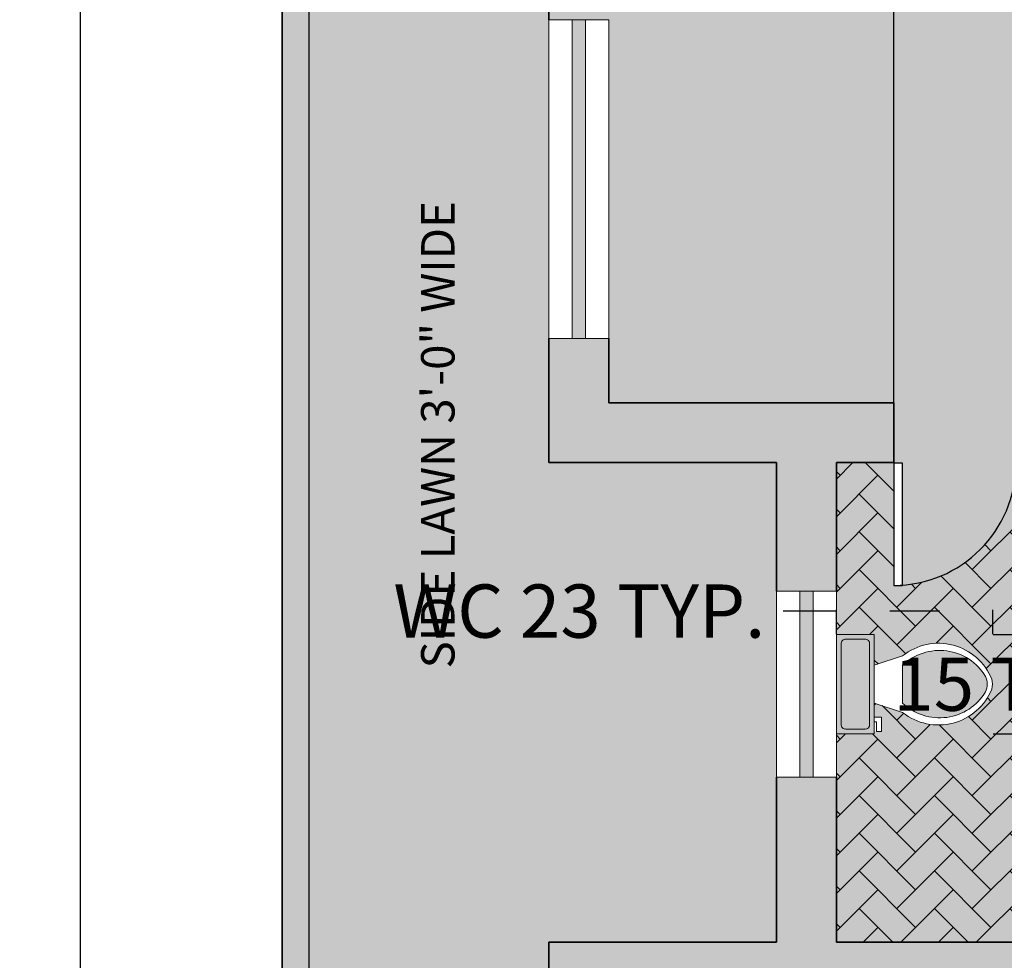
# Model space of a CAD drawing. Units: inches. Extents: x 389 to 971, y 148 to 870.
# Tile 8 of 14: x 389 to 537, y 558 to 699. Entities that reach past the tile are written whole.
import ezdxf

# ---------------------------------------------------------------- set-up
doc = ezdxf.new("R2010")
doc.units = ezdxf.units.IN
doc.header["$MEASUREMENT"] = 0
for name, color, linetype, lineweight in [('A-ANNO-DIMS', 2, 'Continuous', 18), ('A-ANNO-TEXT', 7, 'Continuous', 18), ('A-DOOR', 4, 'Continuous', 25), ('A-FLOR-BASE-PATT', 8, 'Continuous', 13), ('A-FLOR-FIXT', 8, 'Continuous', 18), ('A-FLOR-FIXT-PATT', 9, 'Continuous', 13), ('A-FLOR-PATT', 9, 'Continuous', 13), ('A-GLAZ', 4, 'Continuous', 18), ('A-WALL', 7, 'Continuous', 35), ('C-PROP', 7, 'Continuous', 35), ('L-GRND-BASE-PATT', 8, 'Continuous', 13), ('L-WALL', 7, 'Continuous', 30)]:
    doc.layers.add(name, color=color, linetype=linetype, lineweight=lineweight)
for name, color, linetype, lineweight, true_color in [('A-GLAZ-PATT', 251, 'Continuous', 13, 0x6d5f6c), ('A-WALL-PATT', 18, 'Continuous', 13, 0x000000), ('L-GRND-PATT', 39, 'Continuous', 13, 0x603913)]:
    doc.layers.add(name, color=color, linetype=linetype, lineweight=lineweight, true_color=true_color)
doc.styles.get("Standard").update_dxf_attribs({"font": 'arial.ttf'})
doc.dimstyles.get("Standard").update_dxf_attribs({"dimtxt": 8, "dimasz": 8, "dimexe": 0.18, "dimexo": 0.0625, "dimgap": 0.09, "dimtad": 0, "dimtih": 1, "dimtoh": 1, "dimdec": 0, "dimzin": 0, "dimdsep": 46, "dimlunit": 3, "dimtxsty": 'Standard', "dimcen": 0.09, "dimadec": 0, "dimazin": 0, "dimtfac": 1, "dimtdec": 0, "dimtofl": 0, "dimtmove": 0, "dimatfit": 3, "dimfxl": 1, "dimtolj": 1, "dimtzin": 0, "dimarcsym": 0})

# ---------------------------------------------------------------- blocks, each defined once
blk = doc.blocks.new('*U4')
for p, q in [((0, 0), (0, 6)), ((24, 0), (24, 6))]:
    blk.add_line(p, q)
blk.add_lwpolyline([(0, 0), (0, -24), (1.75, -24), (1.75, 0)], close=True)
blk.add_arc((0, 0), 24, 270, 0)
blk = doc.blocks.new('Toilet - top')
for p, q in [((9.5, -6), (9.5, -2)), ((-8, -8.5), (-8, -8)), ((-7, -8), (-7, -9.5)), ((-4, -8), (-6, -14)), ((4, -8), (6, -14)), ((-10, -8.5), (-8, -8.5)), ((-10, -9.5), (-10, -8.5)), ((-7, -9.5), (-10, -9.5)), ((4, -14), (-4, -14))]:
    blk.add_line(p, q)
blk.add_lwpolyline([(10.5, -8), (10.5, 0), (-10.5, 0), (-10.5, -8)], close=True)
for points in [[(-9.5, -2), (-9.5, -6)], [(8.5, -1), (-8.5, -1)], [(-8.5, -7), (8.5, -7)]]:
    blk.add_lwpolyline(points)
for centre, radius, start, end in [((-8.62, -1.88), 0.884, 81.8699, 188.1301), ((8.62, -1.88), 0.884, 351.8699, 98.1301), ((-8.62, -6.12), 0.884, 171.8699, 278.1301), ((8.62, -6.12), 0.884, 261.8699, 8.1301), ((3.52, -21.58), 12.17, 141.4691, 247.9714), ((4.2, -21.82), 11.33, 136.3677, 238.9468), ((-3.52, -21.58), 12.17, 292.0284, 38.5307), ((-4.2, -21.82), 11.33, 301.053, 43.6321), ((0, -27.88), 4, 245.7318, 294.2682), ((0, -29), 4, 254.8605, 285.1395)]:
    blk.add_arc(centre, radius, start, end)
blk = doc.blocks.new('*D26')
at = {"layer": 'A-ANNO-DIMS', "color": 0, "lineweight": -2, "transparency": 16777216}
for p, q in [((511.39, 610.36), (503.39, 610.36)), ((511.39, 606.91), (511.39, 610.54)), ((526.83, 610.36), (519.39, 610.36)), ((534.83, 606.91), (534.83, 610.54))]:
    blk.add_line(p, q, dxfattribs=at)
at = {"layer": 'A-ANNO-DIMS', "color": 0, "transparency": 16777216}
for points in [[(519.39, 611.69), (519.39, 609.03), (511.39, 610.36)], [(526.83, 611.69), (526.83, 609.03), (534.83, 610.36)]]:
    blk.add_solid(points, dxfattribs=at)
at = {"layer": 'Defpoints', "color": 0, "transparency": 16777216}
for p in [(511.39, 610.36), (511.39, 606.84), (534.83, 606.84)]:
    blk.add_point(p, dxfattribs=at)
at = {"layer": 'A-ANNO-DIMS', "color": 0, "transparency": 16777216, "insert": (472.8, 610.36), "char_height": 8, "attachment_point": 5}
blk.add_mtext('\\A1;WC 23 TYP.', dxfattribs=at)
blk = doc.blocks.new('*D27')
at = {"layer": 'A-ANNO-DIMS', "color": 0, "lineweight": -2, "transparency": 16777216}
for p, q in [((538.35, 614.84), (538.35, 622.84)), ((534.89, 606.84), (538.53, 606.84)), ((534.89, 591.95), (538.53, 591.95)), ((538.35, 583.95), (538.35, 575.95))]:
    blk.add_line(p, q, dxfattribs=at)
at = {"layer": 'A-ANNO-DIMS', "color": 0, "transparency": 16777216}
for points in [[(537.01, 614.84), (539.68, 614.84), (538.35, 606.84)], [(537.01, 583.95), (539.68, 583.95), (538.35, 591.95)]]:
    blk.add_solid(points, dxfattribs=at)
at = {"layer": 'Defpoints', "color": 0, "transparency": 16777216}
for p in [(534.83, 606.84), (538.35, 606.84), (534.83, 591.95)]:
    blk.add_point(p, dxfattribs=at)
at = {"layer": 'A-ANNO-DIMS', "color": 0, "transparency": 16777216, "insert": (538.35, 599.39), "char_height": 8, "attachment_point": 5}
blk.add_mtext('\\A1;15 TYP.', dxfattribs=at)
blk = doc.blocks.new('*D45')
at = {"layer": 'A-ANNO-DIMS', "color": 0, "lineweight": -2, "transparency": 16777216}
for p, q in [((428.15, 834.64), (397.71, 834.64)), ((397.89, 826.64), (397.89, 538.82)), ((397.89, 242.64), (397.89, 530.47)), ((428.15, 234.64), (397.71, 234.64))]:
    blk.add_line(p, q, dxfattribs=at)
at = {"layer": 'A-ANNO-DIMS', "color": 0, "transparency": 16777216}
for points in [[(396.56, 826.64), (399.22, 826.64), (397.89, 834.64)], [(396.56, 242.64), (399.22, 242.64), (397.89, 234.64)]]:
    blk.add_solid(points, dxfattribs=at)
at = {"layer": 'Defpoints', "color": 0, "transparency": 16777216}
for p in [(397.89, 834.64), (428.22, 834.64), (428.22, 234.64)]:
    blk.add_point(p, dxfattribs=at)
at = {"layer": 'A-ANNO-DIMS', "color": 0, "transparency": 16777216, "insert": (397.89, 534.64), "char_height": 8, "attachment_point": 5}
blk.add_mtext('\\A1;600', dxfattribs=at)
blk = doc.blocks.new('*D49')
at = {"layer": 'A-ANNO-DIMS', "color": 0, "lineweight": -2, "transparency": 16777216}
for p, q in [((519.98, 632.71), (519.98, 865.15)), ((527.98, 864.97), (530.32, 864.97)), ((538.32, 632.71), (538.32, 865.15)), ((538.32, 864.97), (546.32, 864.97))]:
    blk.add_line(p, q, dxfattribs=at)
at = {"layer": 'A-ANNO-DIMS', "color": 0, "transparency": 16777216}
for points in [[(527.98, 866.3), (527.98, 863.64), (519.98, 864.97)], [(530.32, 866.3), (530.32, 863.64), (538.32, 864.97)]]:
    blk.add_solid(points, dxfattribs=at)
at = {"layer": 'Defpoints', "color": 0, "transparency": 16777216}
for p in [(538.32, 864.97), (519.98, 632.64), (538.32, 632.64)]:
    blk.add_point(p, dxfattribs=at)
at = {"layer": 'A-ANNO-DIMS', "color": 0, "transparency": 16777216, "insert": (559.52, 864.97), "char_height": 8, "attachment_point": 5}
blk.add_mtext('\\A1;18.34', dxfattribs=at)

msp = doc.modelspace()

# ---------------------------------------------------------------- hatches: boundary and pattern name
at = {"layer": 'A-FLOR-BASE-PATT'}
h = msp.add_hatch(color=256, dxfattribs=at)
h.dxf.hatch_style = 1
h.paths.add_polyline_path([(651.6417, 675.6801), (651.6417, 675.7122), (653.109, 675.7122), (653.109, 641.6445), (661.216, 641.6445), (661.216, 785.6445), (616.7487, 785.6445), (616.7487, 768.9039), (600.0901, 768.9039), (600.0901, 705.6445), (540.0901, 705.6445), (540.0901, 768.9039), (523.3494, 768.9039), (523.3494, 785.6445), (477.216, 785.6445), (477.216, 777.4428), (477.216, 728.9805), (477.216, 699.1491), (477.216, 651.2738), (477.216, 641.6445), (519.983, 641.6445), (519.983, 632.5593), (521.3203, 632.5593), (521.3203, 614.2674, 0.39433689), (538.3235, 632.6445), (538.3237, 632.6445), (538.3237, 637.1445), (538.3237, 641.6445), (619.5719, 641.6445), (619.5719, 642.1751, -0.40145271)])
h.paths.add_polyline_path([(546.1308, 677.2872), (587.0907, 677.2872), (587.0907, 696.0138), (546.1308, 696.0138)], flags=24)
h = msp.add_hatch(color=256, dxfattribs=at)
h.dxf.hatch_style = 1
h.paths.add_polyline_path([(558.5088, 560.6445), (558.5088, 582.7714), (595.387, 582.7714), (595.387, 632.6445), (577.0646, 632.1376, -0.09003216), (582.3048, 631.1863, -0.09001579), (586.1007, 628.9176, -0.10446928), (588.6866, 625.476, -0.11763426), (589.4557, 621.7198, -0.11763426), (588.4463, 618.021, -0.10446928), (585.6443, 614.753, -0.09001579), (581.7102, 612.7333, -0.08191995), (576.8993, 612.0982, -0.08191995), (572.1392, 613.0417, -0.09001579), (568.3432, 615.3105, -0.10446928), (565.7574, 618.7521, -0.11763426), (564.9883, 622.5082, -0.11763426), (565.9976, 626.207, -0.10446928), (568.7997, 629.475, -0.09001579), (572.7338, 631.4947, -0.07381843), (577.0646, 632.1376), (538.3237, 632.6445), (538.3237, 632.5593, -0.39299579), (521.3203, 614.2674), (521.3203, 614.2186), (519.983, 614.2186), (519.983, 632.6445), (511.387, 632.6445), (511.387, 613.354), (511.387, 606.8427), (517.062, 606.8427), (517.062, 602.2317), (521.3182, 603.6504, -0.50132349), (534.6979, 600.1353, -0.13289091), (534.6979, 598.6532, -0.50131678), (521.3183, 595.1379), (517.062, 596.5567), (517.062, 594.4286), (518.1261, 594.4286), (518.1261, 592.3005), (517.062, 592.3005), (517.062, 591.9458), (511.387, 591.9458), (511.387, 585.4344), (511.387, 560.6445)])
h.paths.add_polyline_path([(541.6656, 589.1356), (574.8272, 589.1356), (574.8272, 607.8622), (541.6656, 607.8622)], flags=24)
at = {"layer": 'A-FLOR-FIXT-PATT'}
h = msp.add_hatch(color=256, dxfattribs=at)
h.dxf.hatch_style = 1
h.paths.add_polyline_path([(517.062, 606.8427), (511.387, 606.8427), (511.387, 591.9458), (517.062, 591.9458)])
h.paths.add_polyline_path([(521.3183, 602.2318, -0.4800795), (533.7486, 600.5605, -0.21500378), (533.7486, 598.228, -0.48007965), (521.3183, 596.5568)], flags=17)
at = {"layer": 'A-FLOR-PATT'}
h = msp.add_hatch(dxfattribs=at)
h.set_pattern_fill('AR-HBONE', color=256)
h.paths.add_polyline_path([(521.3183, 595.1379), (517.062, 596.5567), (517.062, 594.4286), (518.1261, 594.4286), (518.1261, 592.3005), (517.062, 592.3005), (517.062, 591.9458), (511.387, 591.9458), (511.387, 585.4344), (511.387, 560.6445), (558.5088, 560.6445), (558.5088, 582.7714), (595.387, 582.7714), (595.387, 632.6445), (577.0646, 632.1376, -0.09003216), (582.3048, 631.1863, -0.09001579), (586.1007, 628.9176, -0.10446928), (588.6866, 625.476, -0.11763426), (589.4557, 621.7198, -0.11763426), (588.4463, 618.021, -0.10446928), (585.6443, 614.753, -0.09001579), (581.7102, 612.7333, -0.08191995), (576.8993, 612.0982, -0.08191995), (572.1392, 613.0417, -0.09001579), (568.3432, 615.3105, -0.10446928), (565.7574, 618.7521, -0.11763426), (564.9883, 622.5082, -0.11763426), (565.9976, 626.207, -0.10446928), (568.7997, 629.475, -0.09001579), (572.7338, 631.4947, -0.07381843), (577.0646, 632.1376), (538.3237, 632.6445), (538.3237, 632.5593, -0.39299579), (521.3203, 614.2674), (521.3203, 614.2186), (519.983, 614.2186), (519.983, 632.6445), (511.387, 632.6445), (511.387, 613.354), (511.387, 606.8427), (517.062, 606.8427), (517.062, 602.2317), (521.3182, 603.6504, -0.50132349), (534.6979, 600.1353, -0.13289091), (534.6979, 598.6532, -0.50131678)])
h.paths.add_polyline_path([(541.6656, 589.1356), (574.8272, 589.1356), (574.8272, 607.8622), (541.6656, 607.8622)], flags=24)
at = {"layer": 'A-GLAZ-PATT'}
h = msp.add_hatch(color=256, dxfattribs=at)
h.dxf.hatch_style = 1
h.paths.add_polyline_path([(473.716, 699.1491), (471.716, 699.1491), (471.716, 651.2738), (473.716, 651.2738)])
h = msp.add_hatch(color=256, dxfattribs=at)
h.dxf.hatch_style = 1
h.paths.add_polyline_path([(505.887, 585.4344), (507.887, 585.4344), (507.887, 613.354), (505.887, 613.354)])
at = {"layer": 'A-WALL-PATT'}
h = msp.add_hatch(color=256, dxfattribs=at)
h.dxf.hatch_style = 1
h.paths.add_polyline_path([(432.216, 434.6445), (436.3673, 434.6445), (436.3673, 443.6445), (432.216, 443.6445), (432.216, 830.6445), (746.216, 830.6445), (746.216, 823.8175), (755.216, 823.8175), (755.216, 825.6445), (839.216, 825.6445), (839.216, 803.5176), (839.216, 741.6445), (755.216, 741.6445), (755.216, 748.4596), (755.1859, 748.4596), (750.716, 748.4596), (746.216, 748.4596), (746.216, 732.6445), (839.216, 732.6445), (839.216, 600.6445), (708.5171, 600.6445), (708.5171, 596.1445), (708.5171, 591.6445), (794.216, 591.6445), (794.216, 587.4291), (803.216, 587.4291), (803.216, 591.6445), (839.216, 591.6445), (839.216, 466.6012), (803.216, 466.6012), (803.216, 471.0309), (794.216, 471.0309), (794.216, 466.6012), (784.6145, 466.6012), (784.6145, 457.6012), (839.216, 457.6012), (839.216, 447.6445), (839.216, 294.6445), (810.0514, 294.6445), (810.0514, 285.6445), (839.216, 285.6445), (839.216, 238.6445), (590.216, 238.6445), (590.216, 234.6445), (848.216, 234.6445), (848.216, 834.6445), (428.216, 834.6445), (428.216, 234.6445), (437.216, 234.6445), (437.216, 243.6445), (432.216, 243.6445)])
h = msp.add_hatch(color=256, dxfattribs=at)
h.dxf.hatch_style = 1
h.paths.add_polyline_path([(468.216, 699.1491), (477.216, 699.1491), (477.216, 728.9805), (468.216, 728.9805)])
h = msp.add_hatch(color=256, dxfattribs=at)
h.dxf.hatch_style = 1
h.paths.add_polyline_path([(502.387, 632.6445), (502.387, 613.354), (511.387, 613.354), (511.387, 632.6445), (519.983, 632.6445), (519.983, 637.1445), (519.983, 641.6445), (477.216, 641.6445), (477.216, 651.2738), (468.216, 651.2738), (468.216, 632.6445)])
h = msp.add_hatch(color=256, dxfattribs=at)
h.dxf.hatch_style = 1
h.paths.add_polyline_path([(538.3237, 641.6445), (538.3237, 637.1445), (538.3237, 632.6445), (595.387, 632.6445), (595.387, 560.6445), (558.5088, 560.6445), (511.387, 560.6445), (511.387, 585.4344), (502.387, 585.4344), (502.387, 560.6445), (468.216, 560.6445), (468.216, 543.0462), (477.216, 543.0462), (477.216, 551.6445), (595.387, 551.6445), (595.387, 545.7317), (595.3894, 545.7317), (599.887, 545.7317), (604.387, 545.7317), (604.387, 632.6445), (619.5147, 632.6445), (619.5147, 641.6445)])
at = {"layer": 'L-GRND-BASE-PATT'}
h = msp.add_hatch(color=256, dxfattribs=at)
h.dxf.hatch_style = 1
h.paths.add_polyline_path([(468.216, 560.6445), (502.387, 560.6445), (502.387, 585.4344), (502.387, 613.354), (502.387, 632.6445), (468.216, 632.6445), (468.216, 651.2738), (468.216, 699.1491), (468.216, 728.9805), (468.216, 777.4428), (468.216, 794.6445), (534.7176, 794.6445), (606.2724, 794.6445), (685.2392, 794.6445), (734.7772, 794.6445), (746.216, 794.6445), (746.216, 796.191), (746.216, 823.8175), (746.216, 830.6445), (432.216, 830.6445), (432.216, 443.6445), (468.216, 443.6445), (468.216, 452.1978), (468.216, 490.1255), (468.216, 508.3496), (468.216, 543.0462)])
h.paths.add_polyline_path([(456.8918, 600.1849), (456.8918, 677.4216), (446.55, 677.4216), (446.55, 600.1849)], flags=24)
h.paths.add_polyline_path([(573.4326, 807.2886), (651.063, 807.2886), (651.063, 817.6304), (573.4326, 817.6304)], flags=24)
at = {"layer": 'L-GRND-PATT'}
h = msp.add_hatch(dxfattribs=at)
h.set_pattern_fill('EARTH', color=256, angle=45)
h.set_pattern_definition([(45, (0, 0), (0, 8.980256), [6.35, -6.35]), (45, (-1.684, 1.684), (0, 8.980256), [6.35, -6.35]), (45, (-3.3676, 3.3676), (0, 8.980256), [6.35, -6.35]), (135, (-3.3676, 4.49), (-8.980256, 0), [6.35, -6.35]), (135, (-1.684, 6.174), (-8.980256, 0), [6.35, -6.35]), (135, (0, 7.858), (-8.980256, 0), [6.35, -6.35])])
h.paths.add_polyline_path([(468.216, 560.6445), (502.387, 560.6445), (502.387, 585.4344), (502.387, 613.354), (502.387, 632.6445), (468.216, 632.6445), (468.216, 651.2738), (468.216, 699.1491), (468.216, 728.9805), (468.216, 777.4428), (468.216, 794.6445), (534.7176, 794.6445), (606.2724, 794.6445), (685.2392, 794.6445), (734.7772, 794.6445), (746.216, 794.6445), (746.216, 796.191), (746.216, 823.8175), (746.216, 830.6445), (432.216, 830.6445), (432.216, 443.6445), (468.216, 443.6445), (468.216, 452.1978), (468.216, 490.1255), (468.216, 508.3496), (468.216, 543.0462)])
h.paths.add_polyline_path([(456.8918, 600.1849), (456.8918, 677.4216), (446.55, 677.4216), (446.55, 600.1849)], flags=24)
h.paths.add_polyline_path([(573.4326, 807.2886), (651.063, 807.2886), (651.063, 817.6304), (573.4326, 817.6304)], flags=24)

# ---------------------------------------------------------------- linework, layer by layer
at = {"layer": 'A-GLAZ'}
for p, q in [((477.216, 699.1491), (468.216, 699.1491)), ((468.216, 699.1491), (468.216, 651.2738)), ((471.716, 699.1491), (471.716, 651.2738)), ((473.716, 699.1491), (473.716, 651.2738)), ((477.216, 699.1491), (477.216, 651.2738)), ((477.216, 651.2738), (468.216, 651.2738)), ((511.387, 613.354), (502.387, 613.354)), ((502.387, 613.354), (502.387, 585.4344)), ((505.887, 613.354), (505.887, 585.4344)), ((507.887, 613.354), (507.887, 585.4344)), ((511.387, 613.354), (511.387, 585.4344)), ((511.387, 585.4344), (502.387, 585.4344))]:
    msp.add_line(p, q, dxfattribs=at)
at = {"layer": 'A-WALL'}
for p, q in [((468.216, 728.9805), (468.216, 699.1491)), ((468.216, 651.2738), (468.216, 632.6445)), ((477.216, 651.2738), (477.216, 641.6445)), ((519.983, 641.6445), (477.216, 641.6445)), ((519.983, 641.6445), (519.983, 632.6445)), ((502.387, 632.6445), (468.216, 632.6445)), ((502.387, 632.6445), (502.387, 613.354)), ((511.387, 632.6445), (511.387, 613.354)), ((519.983, 632.6445), (511.387, 632.6445)), ((502.387, 585.4344), (502.387, 560.6445)), ((511.387, 585.4344), (511.387, 560.6445)), ((468.216, 560.6445), (468.216, 543.0462)), ((502.387, 560.6445), (468.216, 560.6445)), ((595.387, 560.6445), (511.387, 560.6445))]:
    msp.add_line(p, q, dxfattribs=at)
at = {"layer": 'C-PROP'}
msp.add_line((428.216, 834.6445), (428.216, 234.6445), dxfattribs=at)
at = {"layer": 'L-WALL'}
msp.add_line((432.216, 830.6445), (432.216, 443.6445), dxfattribs=at)

# ---------------------------------------------------------------- block references
at = {"layer": 'A-DOOR', "xscale": 0.7641975514951928, "yscale": 0.7641975514951928, "zscale": 0.7641975514951928}
msp.add_blockref('*U4', (519.983, 632.5593), dxfattribs=at)
at = {"layer": 'A-FLOR-FIXT', "xscale": 0.7093753115454805, "yscale": 0.7093753115454805, "zscale": 0.7093753115454805, "rotation": 90}
msp.add_blockref('Toilet - top', (511.387, 599.3942), dxfattribs=at)

# ---------------------------------------------------------------- texts
at = {"layer": 'A-ANNO-TEXT', "insert": (449.0473, 601.7545), "char_height": 5.018573, "attachment_point": 1, "rotation": 90}
msp.add_mtext_dynamic_manual_height_columns('SIDE LAWN 3\'-0" WIDE', width=113.900213, gutter_width=25.0929, heights=[0], dxfattribs=at)

# ---------------------------------------------------------------- dimensions: what is measured, and where the dimension line sits
at = {"layer": 'A-ANNO-DIMS'}
dim = msp.add_linear_dim(base=(538.3237, 864.9695), p1=(519.983, 632.6445), p2=(538.3237, 632.6445), dimstyle='Standard', override={"dimdec": 2, "dimlfac": 1, "dimrnd": 0, "dimzin": 0, "dimdsep": 46, "dimlunit": 2}, dxfattribs=at)
dim.commit()
dim.dimension.update_dxf_attribs({"geometry": '*D49', "text_midpoint": (559.5188, 864.9695)})
dim = msp.add_linear_dim(base=(397.891, 834.6445), p1=(428.216, 234.6445), p2=(428.216, 834.6445), angle=90, dimstyle='Standard', override={"dimdec": 0, "dimlfac": 1, "dimrnd": 0, "dimzin": 0, "dimdsep": 46, "dimlunit": 2}, dxfattribs=at)
dim.commit()
dim.dimension.update_dxf_attribs({"geometry": '*D45', "text_midpoint": (397.891, 534.6445)})
for base, p1, p2, angle, text, picture, middle in [((511.387, 610.359), (534.8292, 606.8427), (511.387, 606.8427), 180, 'WC <> TYP.', '*D26', (472.8004, 610.359)), ((538.3455, 606.8427), (534.8292, 591.9458), (534.8292, 606.8427), 90, '<> TYP.', '*D27', (538.3455, 599.3942))]:
    dim = msp.add_linear_dim(base=base, p1=p1, p2=p2, angle=angle, text=text, dimstyle='Standard', override={"dimdec": 0, "dimlfac": 1, "dimrnd": 0, "dimzin": 0, "dimdsep": 46, "dimlunit": 2}, dxfattribs=at)
    dim.commit()
    dim.dimension.update_dxf_attribs({"geometry": picture, "text_midpoint": middle})

doc.saveas('drawing.dxf')
